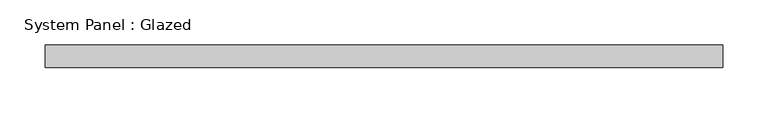
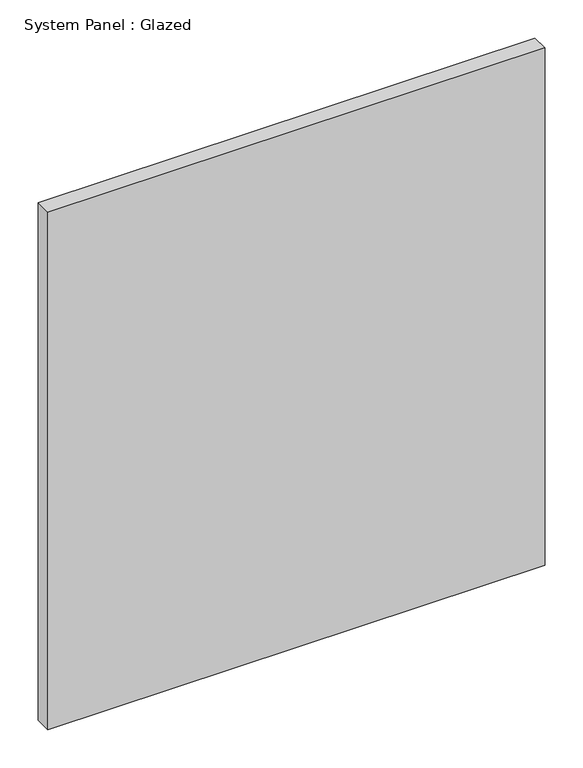
"""IFC4 building model written with IfcOpenShell, lengths in millimetres: plate geometry, System Panel : Glazed."""

from ifc_helpers import new_model, si_unit, origin, origin_with_axes, place, context, project, spatial, polyline, outline, extrude, source, transform, mapped, element, save


def system_panel_glazed_70f3664f(model_context):
    return source(origin(), model_context, "Body", "SweptSolid", [
        extrude(outline(polyline([(375.0, 24.5), (-375.0, 24.5), (-375.0, 49.5), (375.0, 49.5), (375.0, 24.5)])), origin_with_axes(), (0.0, 0.0, 1.0), 825.0),
    ])


if __name__ == "__main__":
    model = new_model("IFC4")
    model_context = context("Model", 3, world=origin())
    ifc_project = project(units=[si_unit("LENGTHUNIT", "METRE", prefix="MILLI")], contexts=[model_context])
    site = spatial("IfcSite", under=ifc_project)
    building = spatial("IfcBuilding", under=site)
    placement = place(None, origin())
    system_panel_glazed_shape = system_panel_glazed_70f3664f(model_context)
    element("IfcPlate", 1, ObjectType="System Panel : Glazed", at=placement, inside=building, context=model_context, shape_type="MappedRepresentation", body=[
        mapped(system_panel_glazed_shape, transform((0.0, 0.0, 0.0), x_axis=(1.0, 0.0, 0.0), y_axis=(0.0, 1.0, 0.0), z_axis=(0.0, 0.0, 1.0))),
    ])
    save(model, "model.ifc")

# Revit data of these elements
# Element 1 (IfcPlate, "System Panel : Glazed")
#   Materials on its faces: "Glass"
# Materials
#   "Glass": class "Glass", colour RGB 218 227 224, transparency 0.85, Description = "Soda Lime Glass", Cost = 0
